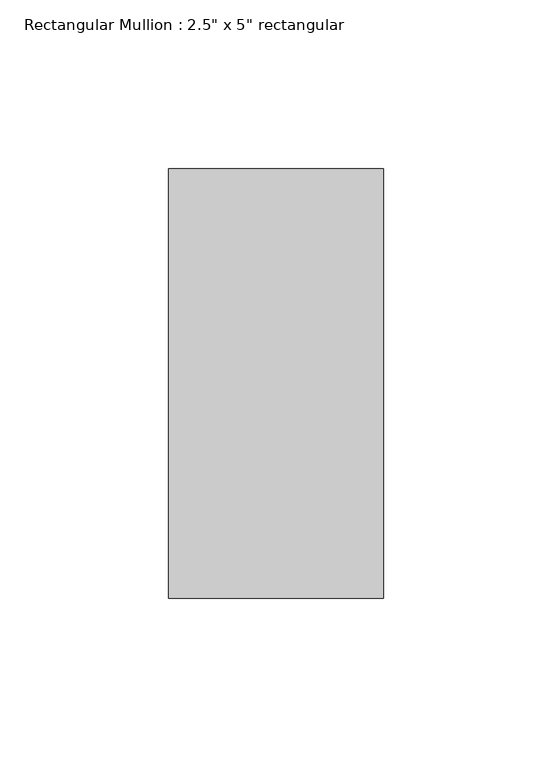
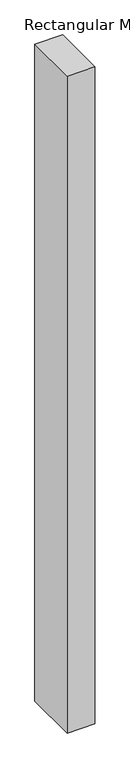
"""IFC4 building model written with IfcOpenShell, lengths in millimetres: member geometry."""

from ifc_helpers import new_model, si_unit, frame, origin, place, context, project, spatial, polyline, outline, extrude, source, transform, mapped, element, save


def member_42ca508f(model_context):
    return source(origin(), model_context, "Body", "SweptSolid", [
        extrude(outline(polyline([(0.0, 63.5), (0.0, -63.5), (-63.5, -63.5), (-63.5, 63.5), (0.0, 63.5)])), frame((0.0, 0.0, -1584.3599864), z_axis=(0.0, 0.0, 1.0), x_axis=(1.0, 0.0, 0.0)), (0.0, 0.0, 1.0), 1584.3599864),
    ])


if __name__ == "__main__":
    model = new_model("IFC4")
    model_context = context("Model", 3, world=origin())
    ifc_project = project(units=[si_unit("LENGTHUNIT", "METRE", prefix="MILLI")], contexts=[model_context])
    site = spatial("IfcSite", under=ifc_project)
    building = spatial("IfcBuilding", under=site)
    placement = place(None, origin())
    member_shape = member_42ca508f(model_context)
    element("IfcMember", 1, ObjectType="Rectangular Mullion : 2.5\" x 5\" rectangular", at=placement, inside=building, context=model_context, shape_type="MappedRepresentation", body=[
        mapped(member_shape, transform((0.0, 0.0, 0.0), x_axis=(1.0, 0.0, 0.0), y_axis=(0.0, 1.0, 0.0), z_axis=(0.0, 0.0, 1.0))),
    ])
    save(model, "model.ifc")

# Revit data of these elements
# Type "Rectangular Mullion : 2.5\" x 5\" rectangular"
#   built-in parameter 1007304 = 0.416667 (stored number, unit not read)
#   built-in parameter 1007301 = 0.104167 (stored number, unit not read)
#   built-in parameter 1007300 = 0.104167 (stored number, unit not read)
# Element 1 (IfcMember, "Rectangular Mullion : 2.5\" x 5\" rectangular")
#   Materials on its faces: "Aluminum"
# Materials
#   "Aluminum": class "Metal", colour RGB 247 247 247, transparency 0, Description = "Aluminum 6061", Cost = 0
